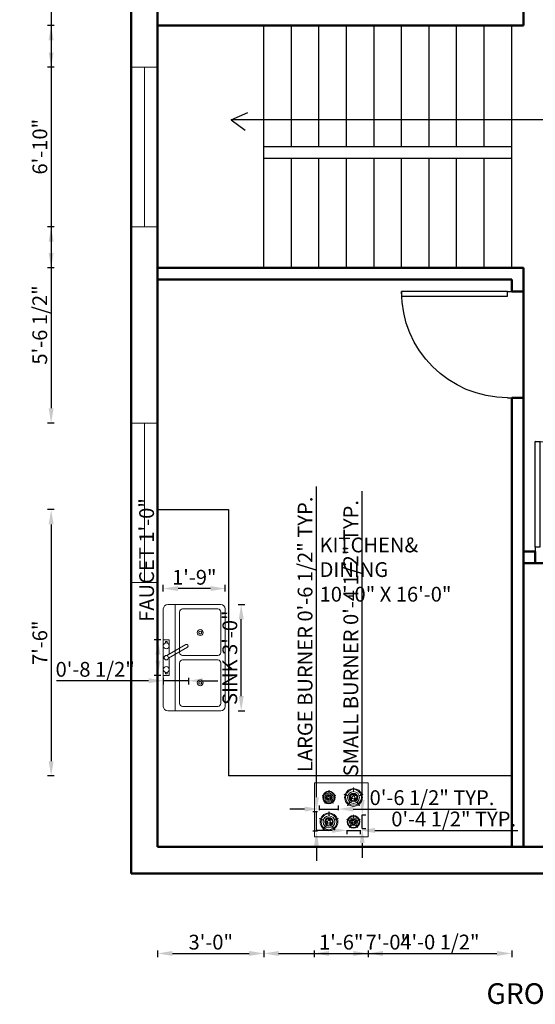
# Model space of a CAD drawing. Units: inches. Extents: x -8 to 396, y -471 to 106.
# Tile 1 of 4: x -8 to 167, y -471 to -138. Entities that reach past the tile are written whole.
import ezdxf

# ---------------------------------------------------------------- set-up
doc = ezdxf.new("R2010")
doc.units = ezdxf.units.IN
for name, color, linetype, lineweight in [('A-ANNO-DIMS', 2, 'Continuous', 18), ('A-ANNO-TEXT', 7, 'Continuous', 25), ('A-AREA-IDEN', 7, 'Continuous', 18), ('A-DOOR', 3, 'Continuous', 25), ('A-EQPM', 8, 'Continuous', 18), ('A-FLOR-CASE', 8, 'Continuous', 25), ('A-FLOR-FIXT', 9, 'Continuous', 18), ('A-FLOR-STRS', 7, 'Continuous', 25), ('A-GLAZ', 4, 'Continuous', 18), ('A-WALL', 7, 'Continuous', 50)]:
    doc.layers.add(name, color=color, linetype=linetype, lineweight=lineweight)
doc.styles.get("Standard").update_dxf_attribs({"font": 'arial.ttf'})
doc.dimstyles.new('ISO-25', dxfattribs={"dimtxt": 5, "dimasz": 5, "dimexe": 1.25, "dimexo": 0.625, "dimtad": 1, "dimlunit": 3, "dimtxsty": 'Standard', "dimcen": 2.5, "dimadec": 0, "dimazin": 0, "dimtfac": 1, "dimtmove": 0, "dimatfit": 3, "dimfxl": 1, "dimfxlon": 1, "dimarcsym": 0})

# ---------------------------------------------------------------- blocks, each defined once
blk = doc.blocks.new('Sink-double - 36 in top')
for p, q in [((-18, -4), (18, -4)), ((-0.75, -18.5), (-0.75, -6.5)), ((0.75, -6.5), (0.75, -18.5))]:
    blk.add_line(p, q)
for points in [[(-16.5, 0), (16.5, 0)], [(-18, -19.5), (-18, -1.5)], [(18, -1.5), (18, -19.5)], [(-16.5, -18.5), (-16.5, -6.5)], [(-15.5, -5.5), (-1.75, -5.5)], [(1.75, -5.5), (15.5, -5.5)], [(16.5, -6.5), (16.5, -18.5)], [(-1.75, -19.5), (-15.5, -19.5)], [(15.5, -19.5), (1.75, -19.5)], [(16.5, -21), (-16.5, -21)]]:
    blk.add_lwpolyline(points)
for centre, radius in [((-8.5, -12.5), 1), ((-8.5, -12.5), 0.5), ((8.5, -12.5), 1), ((8.5, -12.5), 0.5)]:
    blk.add_circle(centre, radius)
for centre, radius, start, end in [((-16.5, -1.5), 1.5, 90, 180), ((16.5, -1.5), 1.5, 0, 90), ((-15.5, -6.5), 1, 90, 180), ((-1.75, -6.5), 1, 0, 90), ((1.75, -6.5), 1, 90, 180), ((15.5, -6.5), 1, 0, 90), ((-16.5, -19.5), 1.5, 180, 270), ((-15.5, -18.5), 1, 180, 270), ((-1.75, -18.5), 1, 270, 0), ((1.75, -18.5), 1, 180, 270), ((15.5, -18.5), 1, 270, 0), ((16.5, -19.5), 1.5, 270, 0)]:
    blk.add_arc(centre, radius, start, end)
blk = doc.blocks.new('Faucet - kit sink top')
for p, q in [((-5.5, -0.75), (-5.5, -1.25)), ((-4.94278, -0.75), (-5.5, -0.75)), ((-5.5, -1.25), (-4.94278, -1.25)), ((-0.14775, -1.7441), (3.56698, -8.1782)), ((4.43301, -7.6782), (0.71828, -1.2441)), ((4.94278, -0.75), (5.5, -0.75)), ((5.5, -1.25), (4.94278, -1.25)), ((5.5, -0.75), (5.5, -1.25))]:
    blk.add_line(p, q)
blk.add_lwpolyline([(-0.00587, -2), (-6, -2), (-6, 0), (6, 0), (6, -2), (1.15195, -2)])
for centre, radius in [((-4, -1), 1), ((4, -1), 1), ((0, -1), 0.75)]:
    blk.add_circle(centre, radius)
blk.add_arc((4, -7.9282), 0.5, 210, 30)
blk = doc.blocks.new('*U5')
for p, q in [((0, 0), (0, -6)), ((40, 0), (40, -6))]:
    blk.add_line(p, q)
blk.add_lwpolyline([(0, 0), (0, 40), (1.75, 40), (1.75, 0)], close=True)
blk.add_arc((0, 0), 40, 0, 90)
blk = doc.blocks.new('WINDOW-54IN')
blk.add_line((4.5, 54), (4.5, 0))
blk.add_lwpolyline([(0, 54), (9, 54), (9, 0), (0, 0)], close=True)
blk = doc.blocks.new('COOKTOP-BURNER-LARGE')
for p, q in [((1.21, 3.59), (0.03, 3.97)), ((1.24, 3.69), (0.07, 4.07)), ((3.13, 5.06), (3.13, 6.29)), ((3.23, 5.06), (3.23, 6.29)), ((5.11, 3.69), (6.29, 4.07)), ((5.15, 3.59), (6.32, 3.97)), ((1.93, 1.37), (1.2, 0.38)), ((2.01, 1.31), (1.28, 0.32)), ((4.34, 1.31), (5.07, 0.32)), ((4.42, 1.37), (5.15, 0.38))]:
    blk.add_line(p, q)
for radius in [2, 1.44, 1.17, 0.501]:
    blk.add_circle((3.18, 3.01), radius)
for centre, radius, start, end in [((0.05, 4.02), 0.0501, 72.0007, 252.0007), ((3.18, 3.01), 3.01, 162.9557, 233.0457), ((3.18, 3.01), 3.01, 90.9557, 161.0457), ((3.18, 3.01), 2.67, 163.075, 232.9263), ((3.18, 3.01), 2.67, 91.075, 160.9263), ((1.22, 3.64), 0.0501, 252.0007, 72.0007), ((3.13, 3.84), 0.167, 93.5265, 273.5265), ((3.18, 3.01), 1, 60.0007, 93.5265), ((3.18, 6.29), 0.0501, 0.0007, 180.0007), ((3.18, 5.06), 0.0501, 180.0007, 0.0007), ((3.18, 3.01), 0.668, 60.0007, 93.5265), ((3.18, 3.01), 3.01, 18.9557, 89.0457), ((3.18, 3.01), 2.67, 19.075, 88.9263), ((3.59, 3.73), 0.167, 240.0007, 60.0007), ((3.18, 3.01), 2.67, 307.075, 16.9263), ((3.18, 3.01), 3.01, 306.9557, 17.0457), ((5.13, 3.64), 0.0501, 108.0007, 288.0007), ((6.3, 4.02), 0.0501, 288.0007, 108.0007), ((1.24, 0.35), 0.0501, 144.0007, 324.0007), ((3.18, 3.01), 3.01, 234.9557, 305.0457), ((3.18, 3.01), 2.67, 235.075, 304.9263), ((1.97, 1.34), 0.0501, 324.0007, 144.0007), ((2.34, 3.01), 0.167, 0.0007, 180.0007), ((3.18, 3.01), 1, 180.0007, 213.5265), ((2.48, 2.54), 0.167, 213.5265, 33.5265), ((3.18, 3.01), 0.668, 180.0007, 213.5265), ((3.59, 2.28), 0.167, 120.0007, 300.0007), ((3.18, 3.01), 0.668, 300.0007, 333.5265), ((3.18, 3.01), 1, 300.0007, 333.5265), ((3.92, 2.63), 0.167, 333.5265, 153.5265), ((4.38, 1.34), 0.0501, 36.0007, 216.0007), ((5.11, 0.35), 0.0501, 216.0007, 36.0007)]:
    blk.add_arc(centre, radius, start, end)
blk = doc.blocks.new('COOKTOP-BURNER-SMALL')
for p, q in [((2.19, 3.54), (2.19, 4.41)), ((2.26, 3.54), (2.26, 4.41)), ((0.85, 2.51), (0.02, 2.78)), ((0.87, 2.58), (0.05, 2.85)), ((1.35, 0.96), (0.84, 0.26)), ((1.41, 0.92), (0.9, 0.22)), ((3.04, 0.92), (3.55, 0.22)), ((3.1, 0.96), (3.6, 0.26)), ((3.58, 2.58), (4.4, 2.85)), ((3.6, 2.51), (4.42, 2.78))]:
    blk.add_line(p, q)
for radius in [1.4, 1.01, 0.818, 0.351]:
    blk.add_circle((2.22, 2.1), radius)
for centre, radius, start, end in [((2.22, 2.1), 2.1, 90.9557, 161.0457), ((2.22, 2.1), 1.87, 91.075, 160.9263), ((2.22, 4.41), 0.0351, 0.0007, 180.0007), ((2.22, 3.54), 0.0351, 180.0007, 0.0007), ((2.22, 2.1), 2.1, 18.9557, 89.0457), ((2.22, 2.1), 1.87, 19.075, 88.9263), ((0.03, 2.81), 0.0351, 72.0007, 252.0007), ((2.22, 2.1), 2.1, 162.9557, 233.0457), ((2.22, 2.1), 1.87, 163.075, 232.9263), ((0.87, 0.24), 0.0351, 144.0007, 324.0007), ((0.86, 2.55), 0.0351, 252.0007, 72.0007), ((2.14, 2.1), 2.1, 234.9557, 305.0457), ((2.22, 2.1), 1.87, 235.075, 304.9263), ((1.38, 0.94), 0.0351, 324.0007, 144.0007), ((1.7, 1.84), 0.117, 26.4748, 206.4748), ((2.22, 2.1), 0.701, 206.4748, 240.0007), ((1.93, 2.61), 0.117, 120.0007, 300.0007), ((2.22, 2.1), 0.468, 206.4748, 240.0007), ((2.22, 2.1), 0.701, 86.4748, 120.0007), ((1.93, 1.6), 0.117, 240.0007, 60.0007), ((2.22, 2.1), 0.468, 86.4748, 120.0007), ((2.26, 2.69), 0.117, 266.4748, 86.4748), ((2.71, 1.78), 0.117, 146.4748, 326.4748), ((2.22, 2.1), 0.468, 326.4748, 0.0007), ((2.81, 2.1), 0.117, 0.0007, 180.0007), ((2.22, 2.1), 0.701, 326.4748, 0.0007), ((3.07, 0.94), 0.0351, 36.0007, 216.0007), ((2.22, 2.1), 1.87, 307.075, 16.9263), ((2.22, 2.1), 2.1, 306.9557, 17.0457), ((3.58, 0.24), 0.0351, 216.0007, 36.0007), ((3.59, 2.55), 0.0351, 108.0007, 288.0007), ((4.41, 2.81), 0.0351, 288.0007, 108.0007)]:
    blk.add_arc(centre, radius, start, end)
blk = doc.blocks.new('*D20')
at = {"layer": 'A-ANNO-DIMS', "color": 0, "lineweight": -2, "transparency": 16777216}
for p, q in [((92.79, -401.06), (92.79, -295.85)), ((93.15, -406.06), (91.54, -406.06)), ((92.79, -412.59), (92.79, -406.06)), ((93.15, -412.59), (91.54, -412.59)), ((92.79, -417.59), (92.79, -422.59))]:
    blk.add_line(p, q, dxfattribs=at)
at = {"layer": 'A-ANNO-DIMS', "color": 0, "transparency": 16777216}
for points in [[(91.96, -401.06), (93.63, -401.06), (92.79, -406.06)], [(91.96, -417.59), (93.63, -417.59), (92.79, -412.59)]]:
    blk.add_solid(points, dxfattribs=at)
at = {"layer": 'Defpoints', "color": 0, "transparency": 16777216}
for p in [(92.79, -406.06), (93.77, -406.06), (93.77, -412.59)]:
    blk.add_point(p, dxfattribs=at)
at = {"layer": 'A-ANNO-DIMS', "color": 0, "transparency": 16777216, "insert": (89.58, -345.95), "char_height": 5, "attachment_point": 5, "rotation": 90}
blk.add_mtext('LARGE BURNER 0\'-6 1/2" TYP.', dxfattribs=at)
blk = doc.blocks.new('*D21')
at = {"layer": 'A-ANNO-DIMS', "color": 0, "lineweight": -2, "transparency": 16777216}
for p, q in [((88.77, -405.08), (83.77, -405.08)), ((93.77, -405.44), (93.77, -403.83)), ((93.77, -405.08), (100.26, -405.08)), ((100.26, -405.44), (100.26, -403.83)), ((105.26, -405.08), (153.64, -405.08))]:
    blk.add_line(p, q, dxfattribs=at)
at = {"layer": 'A-ANNO-DIMS', "color": 0, "transparency": 16777216}
for points in [[(88.77, -404.25), (88.77, -405.91), (93.77, -405.08)], [(105.26, -404.25), (105.26, -405.91), (100.26, -405.08)]]:
    blk.add_solid(points, dxfattribs=at)
at = {"layer": 'Defpoints', "color": 0, "transparency": 16777216}
for p in [(93.77, -406.06), (100.26, -405.08), (100.26, -406.06)]:
    blk.add_point(p, dxfattribs=at)
at = {"layer": 'A-ANNO-DIMS', "color": 0, "transparency": 16777216, "insert": (131.95, -401.87), "char_height": 5, "attachment_point": 5}
blk.add_mtext('0\'-6 1/2" TYP.', dxfattribs=at)
blk = doc.blocks.new('*D22')
at = {"layer": 'A-ANNO-DIMS', "color": 0, "lineweight": -2, "transparency": 16777216}
for p, q in [((108.3, -402.06), (108.3, -297.42)), ((108.24, -407.06), (109.55, -407.06)), ((108.3, -411.63), (108.3, -407.06)), ((108.24, -411.63), (109.55, -411.63)), ((108.3, -416.63), (108.3, -421.63))]:
    blk.add_line(p, q, dxfattribs=at)
at = {"layer": 'A-ANNO-DIMS', "color": 0, "transparency": 16777216}
for points in [[(107.47, -402.06), (109.13, -402.06), (108.3, -407.06)], [(107.47, -416.63), (109.13, -416.63), (108.3, -411.63)]]:
    blk.add_solid(points, dxfattribs=at)
at = {"layer": 'Defpoints', "color": 0, "transparency": 16777216}
for p in [(107.61, -407.06), (108.3, -407.06), (107.61, -411.63)]:
    blk.add_point(p, dxfattribs=at)
at = {"layer": 'A-ANNO-DIMS', "color": 0, "transparency": 16777216, "insert": (105.09, -347.24), "char_height": 5, "attachment_point": 5, "rotation": 90}
blk.add_mtext('SMALL BURNER 0\'-4 1/2" TYP.', dxfattribs=at)
blk = doc.blocks.new('*D23')
at = {"layer": 'A-ANNO-DIMS', "color": 0, "lineweight": -2, "transparency": 16777216}
for p, q in [((98.07, -412.31), (93.07, -412.31)), ((103.07, -412.25), (103.07, -413.56)), ((103.07, -412.31), (107.61, -412.31)), ((107.61, -412.25), (107.61, -413.56)), ((112.61, -412.31), (160.99, -412.31))]:
    blk.add_line(p, q, dxfattribs=at)
at = {"layer": 'A-ANNO-DIMS', "color": 0, "transparency": 16777216}
for points in [[(98.07, -411.48), (98.07, -413.15), (103.07, -412.31)], [(112.61, -411.48), (112.61, -413.15), (107.61, -412.31)]]:
    blk.add_solid(points, dxfattribs=at)
at = {"layer": 'Defpoints', "color": 0, "transparency": 16777216}
for p in [(103.07, -411.63), (107.61, -411.63), (107.61, -412.31)]:
    blk.add_point(p, dxfattribs=at)
at = {"layer": 'A-ANNO-DIMS', "color": 0, "transparency": 16777216, "insert": (139.3, -409.1), "char_height": 5, "attachment_point": 5}
blk.add_mtext('0\'-4 1/2" TYP.', dxfattribs=at)
blk = doc.blocks.new('*D24')
at = {"layer": 'A-ANNO-DIMS', "color": 0, "lineweight": -2, "transparency": 16777216}
for p, q in [((66.29, -335.84), (68.54, -335.84)), ((67.29, -366.84), (67.29, -340.84)), ((66.29, -371.84), (68.54, -371.84))]:
    blk.add_line(p, q, dxfattribs=at)
at = {"layer": 'A-ANNO-DIMS', "color": 0, "transparency": 16777216}
for points in [[(66.46, -340.84), (68.13, -340.84), (67.29, -335.84)], [(66.46, -366.84), (68.13, -366.84), (67.29, -371.84)]]:
    blk.add_solid(points, dxfattribs=at)
at = {"layer": 'Defpoints', "color": 0, "transparency": 16777216}
for p in [(61.89, -335.84), (67.29, -335.84), (61.89, -371.84)]:
    blk.add_point(p, dxfattribs=at)
at = {"layer": 'A-ANNO-DIMS', "color": 0, "transparency": 16777216, "insert": (64.08, -353.84), "char_height": 5, "attachment_point": 5, "rotation": 90}
blk.add_mtext('SINK 3\'-0"', dxfattribs=at)
blk = doc.blocks.new('*D25')
at = {"layer": 'A-ANNO-DIMS', "color": 0, "lineweight": -2, "transparency": 16777216}
for p, q in [((40.89, -331.44), (40.89, -329.19)), ((61.89, -331.44), (61.89, -329.19)), ((56.89, -330.44), (45.89, -330.44))]:
    blk.add_line(p, q, dxfattribs=at)
at = {"layer": 'A-ANNO-DIMS', "color": 0, "transparency": 16777216}
for points in [[(45.89, -329.61), (45.89, -331.28), (40.89, -330.44)], [(56.89, -329.61), (56.89, -331.28), (61.89, -330.44)]]:
    blk.add_solid(points, dxfattribs=at)
at = {"layer": 'Defpoints', "color": 0, "transparency": 16777216}
for p in [(40.89, -330.44), (40.89, -335.84), (61.89, -335.84)]:
    blk.add_point(p, dxfattribs=at)
at = {"layer": 'A-ANNO-DIMS', "color": 0, "transparency": 16777216, "insert": (51.39, -327.27), "char_height": 5, "attachment_point": 5}
blk.add_mtext('1\'-9"', dxfattribs=at)
blk = doc.blocks.new('*D26')
at = {"layer": 'A-ANNO-DIMS', "color": 0, "lineweight": -2, "transparency": 16777216}
for p, q in [((39.09, -347.84), (39.09, -298.7)), ((40.09, -347.84), (37.84, -347.84)), ((39.09, -354.84), (39.09, -352.84)), ((40.09, -359.84), (37.84, -359.84))]:
    blk.add_line(p, q, dxfattribs=at)
at = {"layer": 'A-ANNO-DIMS', "color": 0, "transparency": 16777216}
for points in [[(38.26, -352.84), (39.93, -352.84), (39.09, -347.84)], [(38.26, -354.84), (39.93, -354.84), (39.09, -359.84)]]:
    blk.add_solid(points, dxfattribs=at)
at = {"layer": 'Defpoints', "color": 0, "transparency": 16777216}
for p in [(39.09, -347.84), (40.89, -347.84), (40.89, -359.84)]:
    blk.add_point(p, dxfattribs=at)
at = {"layer": 'A-ANNO-DIMS', "color": 0, "transparency": 16777216, "insert": (35.88, -320.77), "char_height": 5, "attachment_point": 5, "rotation": 90}
blk.add_mtext('FAUCET 1\'-0"', dxfattribs=at)
blk = doc.blocks.new('*D27')
at = {"layer": 'A-ANNO-DIMS', "color": 0, "lineweight": -2, "transparency": 16777216}
for p, q in [((35.89, -361.64), (4.7, -361.64)), ((40.89, -360.64), (40.89, -362.89)), ((49.39, -361.64), (40.89, -361.64)), ((49.39, -360.64), (49.39, -362.89)), ((54.39, -361.64), (59.39, -361.64))]:
    blk.add_line(p, q, dxfattribs=at)
at = {"layer": 'A-ANNO-DIMS', "color": 0, "transparency": 16777216}
for points in [[(35.89, -360.81), (35.89, -362.48), (40.89, -361.64)], [(54.39, -360.81), (54.39, -362.48), (49.39, -361.64)]]:
    blk.add_solid(points, dxfattribs=at)
at = {"layer": 'Defpoints', "color": 0, "transparency": 16777216}
for p in [(40.89, -359.84), (49.39, -359.84), (40.89, -361.64)]:
    blk.add_point(p, dxfattribs=at)
at = {"layer": 'A-ANNO-DIMS', "color": 0, "transparency": 16777216, "insert": (17.8, -358.43), "char_height": 5, "attachment_point": 5}
blk.add_mtext('0\'-8 1/2"', dxfattribs=at)
blk = doc.blocks.new('*D29')
at = {"layer": 'A-ANNO-DIMS', "color": 0, "lineweight": -2, "transparency": 16777216}
for p, q in [((3.88, -85.66), (1.63, -85.66)), ((2.88, -90.66), (2.88, -149)), ((3.88, -154), (1.63, -154))]:
    blk.add_line(p, q, dxfattribs=at)
at = {"layer": 'A-ANNO-DIMS', "color": 0, "transparency": 16777216}
for points in [[(2.04, -90.66), (3.71, -90.66), (2.88, -85.66)], [(2.04, -149), (3.71, -149), (2.88, -154)]]:
    blk.add_solid(points, dxfattribs=at)
at = {"layer": 'Defpoints', "color": 0, "transparency": 16777216}
for p in [(29.97, -85.66), (2.88, -154), (29.97, -154)]:
    blk.add_point(p, dxfattribs=at)
at = {"layer": 'A-ANNO-DIMS', "color": 0, "transparency": 16777216, "insert": (-0.33, -119.83), "char_height": 5, "attachment_point": 5, "rotation": 90}
blk.add_mtext('5\'-8 1/2"', dxfattribs=at)
blk = doc.blocks.new('*D30')
at = {"layer": 'A-ANNO-DIMS', "color": 0, "lineweight": -2, "transparency": 16777216}
for p, q in [((3.88, -208), (1.63, -208)), ((2.88, -213), (2.88, -269.43)), ((3.88, -274.43), (1.63, -274.43))]:
    blk.add_line(p, q, dxfattribs=at)
at = {"layer": 'A-ANNO-DIMS', "color": 0, "transparency": 16777216}
for points in [[(2.04, -213), (3.71, -213), (2.88, -208)], [(2.04, -269.43), (3.71, -269.43), (2.88, -274.43)]]:
    blk.add_solid(points, dxfattribs=at)
at = {"layer": 'Defpoints', "color": 0, "transparency": 16777216}
for p in [(29.97, -208), (2.88, -274.43), (29.97, -274.43)]:
    blk.add_point(p, dxfattribs=at)
at = {"layer": 'A-ANNO-DIMS', "color": 0, "transparency": 16777216, "insert": (-0.33, -241.21), "char_height": 5, "attachment_point": 5, "rotation": 90}
blk.add_mtext('5\'-6 1/2"', dxfattribs=at)
blk = doc.blocks.new('*D34')
at = {"layer": 'A-ANNO-DIMS', "color": 0, "lineweight": -2, "transparency": 16777216}
for p, q in [((3.88, -139.87), (1.63, -139.87)), ((2.88, -144.87), (2.88, -216.87)), ((3.88, -221.87), (1.63, -221.87))]:
    blk.add_line(p, q, dxfattribs=at)
at = {"layer": 'A-ANNO-DIMS', "color": 0, "transparency": 16777216}
for points in [[(2.04, -144.87), (3.71, -144.87), (2.88, -139.87)], [(2.04, -216.87), (3.71, -216.87), (2.88, -221.87)]]:
    blk.add_solid(points, dxfattribs=at)
at = {"layer": 'Defpoints', "color": 0, "transparency": 16777216}
for p in [(38.97, -139.87), (2.88, -221.87), (38.97, -221.87)]:
    blk.add_point(p, dxfattribs=at)
at = {"layer": 'A-ANNO-DIMS', "color": 0, "transparency": 16777216, "insert": (-0.3, -180.87), "char_height": 5, "attachment_point": 5, "rotation": 90}
blk.add_mtext('6\'-10"', dxfattribs=at)
blk = doc.blocks.new('*D35')
at = {"layer": 'A-ANNO-DIMS', "color": 0, "lineweight": -2, "transparency": 16777216}
for p, q in [((74.97, -452.96), (74.97, -455.21)), ((158.97, -452.96), (158.97, -455.21)), ((79.97, -453.96), (153.97, -453.96))]:
    blk.add_line(p, q, dxfattribs=at)
at = {"layer": 'A-ANNO-DIMS', "color": 0, "transparency": 16777216}
for points in [[(79.97, -453.13), (79.97, -454.8), (74.97, -453.96)], [(153.97, -453.13), (153.97, -454.8), (158.97, -453.96)]]:
    blk.add_solid(points, dxfattribs=at)
at = {"layer": 'Defpoints', "color": 0, "transparency": 16777216}
for p in [(74.97, -221.87), (158.97, -221.87), (158.97, -453.96)]:
    blk.add_point(p, dxfattribs=at)
at = {"layer": 'A-ANNO-DIMS', "color": 0, "transparency": 16777216, "insert": (116.97, -450.79), "char_height": 5, "attachment_point": 5}
blk.add_mtext('7\'-0"', dxfattribs=at)
blk = doc.blocks.new('*D36')
at = {"layer": 'A-ANNO-DIMS', "color": 0, "lineweight": -2, "transparency": 16777216}
for p, q in [((38.97, -452.96), (38.97, -455.21)), ((74.97, -452.96), (74.97, -455.21)), ((43.97, -453.96), (69.97, -453.96))]:
    blk.add_line(p, q, dxfattribs=at)
at = {"layer": 'A-ANNO-DIMS', "color": 0, "transparency": 16777216}
for points in [[(43.97, -453.13), (43.97, -454.8), (38.97, -453.96)], [(69.97, -453.13), (69.97, -454.8), (74.97, -453.96)]]:
    blk.add_solid(points, dxfattribs=at)
at = {"layer": 'Defpoints', "color": 0, "transparency": 16777216}
for p in [(38.97, -221.87), (74.97, -221.87), (74.97, -453.96)]:
    blk.add_point(p, dxfattribs=at)
at = {"layer": 'A-ANNO-DIMS', "color": 0, "transparency": 16777216, "insert": (56.97, -450.78), "char_height": 5, "attachment_point": 5}
blk.add_mtext('3\'-0"', dxfattribs=at)
blk = doc.blocks.new('*D37')
at = {"layer": 'A-ANNO-DIMS', "color": 0, "lineweight": -2, "transparency": 16777216}
for p, q in [((380.06, -184.87), (382.31, -184.87)), ((381.06, -216.87), (381.06, -189.87)), ((380.06, -221.87), (382.31, -221.87))]:
    blk.add_line(p, q, dxfattribs=at)
at = {"layer": 'A-ANNO-DIMS', "color": 0, "transparency": 16777216}
for points in [[(380.22, -189.87), (381.89, -189.87), (381.06, -184.87)], [(380.22, -216.87), (381.89, -216.87), (381.06, -221.87)]]:
    blk.add_solid(points, dxfattribs=at)
at = {"layer": 'Defpoints', "color": 0, "transparency": 16777216}
for p in [(158.97, -184.87), (381.06, -184.87), (158.97, -221.87)]:
    blk.add_point(p, dxfattribs=at)
at = {"layer": 'A-ANNO-DIMS', "color": 0, "transparency": 16777216, "insert": (377.88, -203.37), "char_height": 5, "attachment_point": 5, "rotation": 90}
blk.add_mtext('3\'-1"', dxfattribs=at)
blk = doc.blocks.new('*D38')
at = {"layer": 'A-ANNO-DIMS', "color": 0, "lineweight": -2, "transparency": 16777216}
for p, q in [((380.06, -139.87), (382.31, -139.87)), ((381.06, -144.87), (381.06, -175.87)), ((380.06, -180.87), (382.31, -180.87))]:
    blk.add_line(p, q, dxfattribs=at)
at = {"layer": 'A-ANNO-DIMS', "color": 0, "transparency": 16777216}
for points in [[(380.22, -144.87), (381.89, -144.87), (381.06, -139.87)], [(380.22, -175.87), (381.89, -175.87), (381.06, -180.87)]]:
    blk.add_solid(points, dxfattribs=at)
at = {"layer": 'Defpoints', "color": 0, "transparency": 16777216}
for p in [(158.97, -139.87), (158.97, -180.87), (381.06, -180.87)]:
    blk.add_point(p, dxfattribs=at)
at = {"layer": 'A-ANNO-DIMS', "color": 0, "transparency": 16777216, "insert": (377.88, -160.37), "char_height": 5, "attachment_point": 5, "rotation": 90}
blk.add_mtext('3\'-5"', dxfattribs=at)
blk = doc.blocks.new('*D39')
at = {"layer": 'A-ANNO-DIMS', "color": 0, "lineweight": -2, "transparency": 16777216}
for p, q in [((69.97, 95.22), (64.97, 95.22)), ((74.97, 94.22), (74.97, 96.47)), ((74.97, 95.22), (84.3, 95.22)), ((84.3, 94.22), (84.3, 96.47)), ((89.3, 95.22), (120.49, 95.22))]:
    blk.add_line(p, q, dxfattribs=at)
at = {"layer": 'A-ANNO-DIMS', "color": 0, "transparency": 16777216}
for points in [[(69.97, 96.05), (69.97, 94.38), (74.97, 95.22)], [(89.3, 96.05), (89.3, 94.38), (84.3, 95.22)]]:
    blk.add_solid(points, dxfattribs=at)
at = {"layer": 'Defpoints', "color": 0, "transparency": 16777216}
for p in [(84.3, 95.22), (74.97, -139.87), (84.3, -139.87)]:
    blk.add_point(p, dxfattribs=at)
at = {"layer": 'A-ANNO-DIMS', "color": 0, "transparency": 16777216, "insert": (107.39, 98.43), "char_height": 5, "attachment_point": 5}
blk.add_mtext('0\'-9 1/2"', dxfattribs=at)
blk = doc.blocks.new('*D40')
at = {"layer": 'A-ANNO-DIMS', "color": 0, "lineweight": -2, "transparency": 16777216}
for p, q in [((38.97, 94.22), (38.97, 96.47)), ((43.97, 95.22), (57.97, 95.22)), ((62.97, 94.22), (62.97, 96.47))]:
    blk.add_line(p, q, dxfattribs=at)
at = {"layer": 'A-ANNO-DIMS', "color": 0, "transparency": 16777216}
for points in [[(43.97, 96.05), (43.97, 94.38), (38.97, 95.22)], [(57.97, 96.05), (57.97, 94.38), (62.97, 95.22)]]:
    blk.add_solid(points, dxfattribs=at)
at = {"layer": 'Defpoints', "color": 0, "transparency": 16777216}
for p in [(62.97, 95.22), (38.97, -303.72), (62.97, -303.72)]:
    blk.add_point(p, dxfattribs=at)
at = {"layer": 'A-ANNO-DIMS', "color": 0, "transparency": 16777216, "insert": (50.97, 98.39), "char_height": 5, "attachment_point": 5}
blk.add_mtext('2\'-0"', dxfattribs=at)
blk = doc.blocks.new('*D41')
at = {"layer": 'A-ANNO-DIMS', "color": 0, "lineweight": -2, "transparency": 16777216}
for p, q in [((3.88, -303.72), (1.63, -303.72)), ((2.88, -308.72), (2.88, -388.88)), ((3.88, -393.88), (1.63, -393.88))]:
    blk.add_line(p, q, dxfattribs=at)
at = {"layer": 'A-ANNO-DIMS', "color": 0, "transparency": 16777216}
for points in [[(2.04, -308.72), (3.71, -308.72), (2.88, -303.72)], [(2.04, -388.88), (3.71, -388.88), (2.88, -393.88)]]:
    blk.add_solid(points, dxfattribs=at)
at = {"layer": 'Defpoints', "color": 0, "transparency": 16777216}
for p in [(38.97, -303.72), (2.88, -393.88), (62.97, -393.88)]:
    blk.add_point(p, dxfattribs=at)
at = {"layer": 'A-ANNO-DIMS', "color": 0, "transparency": 16777216, "insert": (-0.3, -348.8), "char_height": 5, "attachment_point": 5, "rotation": 90}
blk.add_mtext('7\'-6"', dxfattribs=at)
blk = doc.blocks.new('*D42')
at = {"layer": 'A-ANNO-DIMS', "color": 0, "lineweight": -2, "transparency": 16777216}
for p, q in [((380.06, -303.72), (382.31, -303.72)), ((381.06, -308.72), (381.06, -330.84)), ((380.06, -335.84), (382.31, -335.84))]:
    blk.add_line(p, q, dxfattribs=at)
at = {"layer": 'A-ANNO-DIMS', "color": 0, "transparency": 16777216}
for points in [[(380.22, -308.72), (381.89, -308.72), (381.06, -303.72)], [(380.22, -330.84), (381.89, -330.84), (381.06, -335.84)]]:
    blk.add_solid(points, dxfattribs=at)
at = {"layer": 'Defpoints', "color": 0, "transparency": 16777216}
for p in [(62.97, -303.72), (60.39, -335.84), (381.06, -335.84)]:
    blk.add_point(p, dxfattribs=at)
at = {"layer": 'A-ANNO-DIMS', "color": 0, "transparency": 16777216, "insert": (377.88, -319.78), "char_height": 5, "attachment_point": 5, "rotation": 90}
blk.add_mtext('2\'-8"', dxfattribs=at)
blk = doc.blocks.new('*D43')
at = {"layer": 'A-ANNO-DIMS', "color": 0, "lineweight": -2, "transparency": 16777216}
for p, q in [((92.07, -452.96), (92.07, -455.21)), ((110.29, -452.96), (110.29, -455.21)), ((97.07, -453.96), (105.29, -453.96))]:
    blk.add_line(p, q, dxfattribs=at)
at = {"layer": 'A-ANNO-DIMS', "color": 0, "transparency": 16777216}
for points in [[(97.07, -453.13), (97.07, -454.8), (92.07, -453.96)], [(105.29, -453.13), (105.29, -454.8), (110.29, -453.96)]]:
    blk.add_solid(points, dxfattribs=at)
at = {"layer": 'Defpoints', "color": 0, "transparency": 16777216}
for p in [(92.07, -414.44), (110.29, -414.44), (110.29, -453.96)]:
    blk.add_point(p, dxfattribs=at)
at = {"layer": 'A-ANNO-DIMS', "color": 0, "transparency": 16777216, "insert": (101.18, -450.79), "char_height": 5, "attachment_point": 5}
blk.add_mtext('1\'-6"', dxfattribs=at)
blk = doc.blocks.new('*D44')
at = {"layer": 'A-ANNO-DIMS', "color": 0, "lineweight": -2, "transparency": 16777216}
for p, q in [((380.06, -396.22), (382.31, -396.22)), ((381.06, -409.44), (381.06, -401.22)), ((380.06, -414.44), (382.31, -414.44))]:
    blk.add_line(p, q, dxfattribs=at)
at = {"layer": 'A-ANNO-DIMS', "color": 0, "transparency": 16777216}
for points in [[(380.22, -401.22), (381.89, -401.22), (381.06, -396.22)], [(380.22, -409.44), (381.89, -409.44), (381.06, -414.44)]]:
    blk.add_solid(points, dxfattribs=at)
at = {"layer": 'Defpoints', "color": 0, "transparency": 16777216}
for p in [(110.29, -396.22), (381.06, -396.22), (110.29, -414.44)]:
    blk.add_point(p, dxfattribs=at)
at = {"layer": 'A-ANNO-DIMS', "color": 0, "transparency": 16777216, "insert": (377.88, -405.33), "char_height": 5, "attachment_point": 5, "rotation": 90}
blk.add_mtext('1\'-6"', dxfattribs=at)
blk = doc.blocks.new('*D51')
at = {"layer": 'A-ANNO-DIMS', "color": 0, "lineweight": -2, "transparency": 16777216}
for p, q in [((110.29, -452.96), (110.29, -455.21)), ((158.97, -452.96), (158.97, -455.21)), ((115.29, -453.96), (153.97, -453.96))]:
    blk.add_line(p, q, dxfattribs=at)
at = {"layer": 'A-ANNO-DIMS', "color": 0, "transparency": 16777216}
for points in [[(115.29, -453.13), (115.29, -454.8), (110.29, -453.96)], [(153.97, -453.13), (153.97, -454.8), (158.97, -453.96)]]:
    blk.add_solid(points, dxfattribs=at)
at = {"layer": 'Defpoints', "color": 0, "transparency": 16777216}
for p in [(110.29, -414.44), (158.97, -417.87), (158.97, -453.96)]:
    blk.add_point(p, dxfattribs=at)
at = {"layer": 'A-ANNO-DIMS', "color": 0, "transparency": 16777216, "insert": (134.63, -450.75), "char_height": 5, "attachment_point": 5}
blk.add_mtext('4\'-0 1/2"', dxfattribs=at)

msp = doc.modelspace()

# ---------------------------------------------------------------- linework, layer by layer
at = {"layer": 'A-EQPM'}
msp.add_lwpolyline([(92.071, -414.441), (110.289, -414.441), (110.289, -396.223), (92.071, -396.223)], close=True, dxfattribs=at)
at = {"layer": 'A-FLOR-CASE'}
for p, q in [((38.966, -303.723), (62.966, -303.723)), ((62.966, -303.723), (62.966, -393.88)), ((158.506, -393.88), (62.966, -393.88))]:
    msp.add_line(p, q, dxfattribs=at)
at = {"layer": 'A-FLOR-STRS'}
for p, q in [((74.966, -180.874), (74.966, -139.874)), ((84.299, -180.874), (84.299, -139.874)), ((93.632, -180.874), (93.632, -139.874)), ((102.966, -180.874), (102.966, -139.874)), ((112.299, -180.874), (112.299, -139.874)), ((121.632, -180.874), (121.632, -139.874)), ((130.966, -180.874), (130.966, -139.874)), ((140.299, -180.874), (140.299, -139.874)), ((149.632, -180.874), (149.632, -139.874)), ((158.966, -221.874), (158.966, -139.874)), ((158.966, -180.874), (158.966, -139.874)), ((63.931, -171.819), (69.488, -169.334)), ((177.259, -171.819), (63.931, -171.819)), ((63.931, -171.819), (68.575, -175.302)), ((158.966, -180.874), (74.966, -180.874)), ((74.966, -184.874), (74.966, -180.874)), ((158.966, -184.874), (74.966, -184.874)), ((74.966, -221.874), (74.966, -184.874)), ((84.299, -221.874), (84.299, -184.874)), ((93.632, -221.874), (93.632, -184.874)), ((102.966, -221.874), (102.966, -184.874)), ((112.299, -221.874), (112.299, -184.874)), ((121.632, -221.874), (121.632, -184.874)), ((130.966, -221.874), (130.966, -184.874)), ((140.299, -221.874), (140.299, -184.874)), ((149.632, -221.874), (149.632, -184.874)), ((158.966, -221.874), (158.966, -184.874))]:
    msp.add_line(p, q, dxfattribs=at)
at = {"layer": 'A-WALL'}
for p, q in [((29.966, -426.874), (29.966, 17.126)), ((38.966, -139.874), (38.966, 8.126)), ((162.966, -139.874), (162.966, 8.126)), ((38.966, -139.874), (162.966, -139.874)), ((38.966, -225.874), (38.966, -139.874)), ((158.966, -221.874), (38.966, -221.874)), ((158.966, -221.874), (162.966, -221.874)), ((162.966, -417.874), (162.966, -221.874)), ((38.966, -417.874), (38.966, -225.874)), ((158.966, -225.874), (38.966, -225.874)), ((158.966, -229.874), (158.966, -225.874)), ((158.966, -229.874), (162.966, -229.874)), ((158.966, -417.874), (158.966, -265.874)), ((158.966, -265.874), (162.966, -265.874)), ((166.966, -317.874), (162.966, -317.874)), ((166.966, -317.874), (166.966, -321.874)), ((218.966, -321.874), (162.966, -321.874)), ((158.966, -417.874), (38.966, -417.874)), ((162.966, -417.874), (158.966, -417.874)), ((218.966, -417.874), (162.966, -417.874)), ((353.966, -426.874), (29.966, -426.874))]:
    msp.add_line(p, q, dxfattribs=at)

# ---------------------------------------------------------------- block references
at = {"layer": 'A-DOOR', "xscale": -0.8988723868321489, "yscale": 0.8988723868321489, "zscale": 0.8988723868321489, "rotation": 90}
msp.add_blockref('*U5', (157.572, -229.874), dxfattribs=at)
at = {"layer": 'A-DOOR', "xscale": 0.894851635990925, "yscale": 0.894851635990925, "zscale": 0.894851635990925}
msp.add_blockref('*U5', (166.966, -316.451), dxfattribs=at)
at = {"layer": 'A-EQPM'}
for name, p in [('COOKTOP-BURNER-SMALL', (94.793, -403.261)), ('COOKTOP-BURNER-LARGE', (102.167, -404.163)), ('COOKTOP-BURNER-LARGE', (93.84, -412.404)), ('COOKTOP-BURNER-SMALL', (103.12, -411.502))]:
    msp.add_blockref(name, p, dxfattribs=at)
at = {"layer": 'A-FLOR-FIXT', "rotation": 90}
for name in ['Sink-double - 36 in top', 'Faucet - kit sink top']:
    msp.add_blockref(name, (40.893, -353.844), dxfattribs=at)
at = {"layer": 'A-GLAZ'}
for p in [(29.966, -207.998), (29.966, -328.426)]:
    msp.add_blockref('WINDOW-54IN', p, dxfattribs=at)

# ---------------------------------------------------------------- texts
at = {"layer": 'A-ANNO-TEXT', "insert": (150.401, -464.054), "char_height": 7, "attachment_point": 1}
msp.add_mtext_dynamic_manual_height_columns('GROUND FLOOR PLAN', width=215.36302, gutter_width=12.5, heights=[0], dxfattribs=at)
at = {"layer": 'A-AREA-IDEN', "insert": (93.859, -313.188), "char_height": 5, "attachment_point": 1}
msp.add_mtext_dynamic_manual_height_columns('KITCHEN& DINING\\P10\'-0" X 16\'-0"', width=45.45203, gutter_width=12.5, heights=[0], dxfattribs=at)

# ---------------------------------------------------------------- dimensions: what is measured, and where the dimension line sits
at = {"layer": 'A-ANNO-DIMS'}
for base, p1, p2, picture, middle in [((84.299, 95.216), (74.966, -139.874), (84.299, -139.874), '*D39', (107.395, 98.426)), ((62.966, 95.216), (38.966, -303.723), (62.966, -303.723), '*D40', (50.966, 98.394)), ((74.966, -453.964), (38.966, -221.874), (74.966, -221.874), '*D36', (56.966, -450.784)), ((158.966, -453.964), (74.966, -221.874), (158.966, -221.874), '*D35', (116.966, -450.786)), ((110.289, -453.964), (92.071, -414.441), (110.289, -414.441), '*D43', (101.18, -450.786)), ((158.966, -453.964), (110.289, -414.441), (158.966, -417.874), '*D51', (134.627, -450.754))]:
    dim = msp.add_linear_dim(base=base, p1=p1, p2=p2, dimstyle='ISO-25', override={"dimdec": 1, "dimlfac": 1, "dimrnd": 0, "dimzin": 1, "dimdsep": 46, "dimlunit": 4, "dimfrac": 2}, dxfattribs=at)
    dim.commit()
    dim.dimension.update_dxf_attribs({"geometry": picture, "text_midpoint": middle})
for base, p1, p2, angle, picture, middle in [((2.876, -153.998), (29.966, -85.659), (29.966, -153.998), 90, '*D29', (-0.335, -119.828)), ((2.876, -221.874), (38.966, -139.874), (38.966, -221.874), 90, '*D34', (-0.302, -180.874)), ((381.056, -180.874), (158.966, -139.874), (158.966, -180.874), 90, '*D38', (377.876, -160.374)), ((381.056, -184.874), (158.966, -221.874), (158.966, -184.874), 90, '*D37', (377.876, -203.374)), ((2.876, -274.426), (29.966, -207.998), (29.966, -274.426), 90, '*D30', (-0.335, -241.212)), ((2.876, -393.88), (38.966, -303.723), (62.966, -393.88), 90, '*D41', (-0.302, -348.801)), ((381.056, -335.844), (62.966, -303.723), (60.393, -335.844), 90, '*D42', (377.878, -319.783)), ((40.893, -330.444), (61.893, -335.844), (40.893, -335.844), 180, '*D25', (51.393, -327.266)), ((40.893, -361.644), (49.392, -359.844), (40.893, -359.844), 180, '*D27', (17.797, -358.433)), ((381.056, -396.223), (110.289, -414.441), (110.289, -396.223), 90, '*D44', (377.878, -405.332))]:
    dim = msp.add_linear_dim(base=base, p1=p1, p2=p2, angle=angle, dimstyle='ISO-25', override={"dimdec": 1, "dimlfac": 1, "dimrnd": 0, "dimzin": 1, "dimdsep": 46, "dimlunit": 4, "dimfrac": 2}, dxfattribs=at)
    dim.commit()
    dim.dimension.update_dxf_attribs({"geometry": picture, "text_midpoint": middle})
for base, p1, p2, text, picture, middle in [((92.793, -406.06), (93.772, -412.586), (93.772, -406.06), 'LARGE BURNER <> TYP.', '*D20', (89.583, -345.954)), ((39.093, -347.844), (40.893, -359.844), (40.893, -347.844), 'FAUCET <>', '*D26', (35.883, -320.774)), ((108.3, -407.062), (107.615, -411.629), (107.615, -407.062), 'SMALL BURNER <> TYP.', '*D22', (105.09, -347.243)), ((67.293, -335.844), (61.893, -371.844), (61.893, -335.844), 'SINK <>', '*D24', (64.081, -353.844))]:
    dim = msp.add_linear_dim(base=base, p1=p1, p2=p2, angle=90, text=text, dimstyle='ISO-25', override={"dimdec": 1, "dimlfac": 1, "dimrnd": 0, "dimzin": 1, "dimdsep": 46, "dimlunit": 4, "dimfrac": 2}, dxfattribs=at)
    dim.commit()
    dim.dimension.update_dxf_attribs({"geometry": picture, "text_midpoint": middle})
for base, p1, p2, picture, middle in [((100.262, -405.081), (93.772, -406.06), (100.262, -406.06), '*D21', (131.951, -401.871)), ((107.615, -412.315), (103.072, -411.629), (107.615, -411.629), '*D23', (139.304, -409.104))]:
    dim = msp.add_linear_dim(base=base, p1=p1, p2=p2, text='<> TYP.', dimstyle='ISO-25', override={"dimdec": 1, "dimlfac": 1, "dimrnd": 0, "dimzin": 1, "dimdsep": 46, "dimlunit": 4, "dimfrac": 2}, dxfattribs=at)
    dim.commit()
    dim.dimension.update_dxf_attribs({"geometry": picture, "text_midpoint": middle})

doc.saveas('drawing.dxf')
